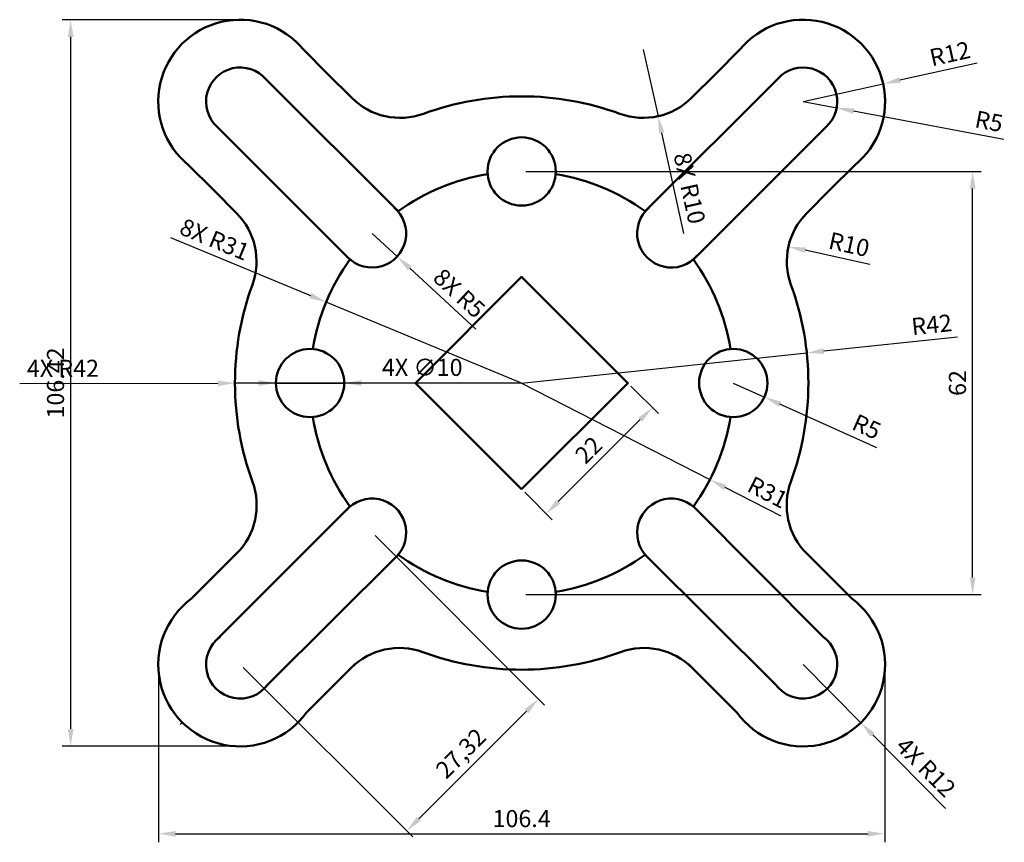
# Model space of a CAD drawing. Units: millimetres. Extents: x 2938 to 3083, y 1829 to 1950.
import ezdxf

# ---------------------------------------------------------------- set-up
doc = ezdxf.new("R2010")
doc.units = ezdxf.units.MM
for name, color, linetype, lineweight in [('M-CONS', 8, 'Continuous', 18), ('M-DIMS', 2, 'Continuous', 25), ('M-OUTL', 7, 'Continuous', 50)]:
    doc.layers.add(name, color=color, linetype=linetype, lineweight=lineweight)
doc.styles.get("Standard").update_dxf_attribs({"font": 'arial.ttf'})
doc.dimstyles.new('ISO-25', dxfattribs={"dimtxt": 2.5, "dimasz": 2.5, "dimexe": 1.25, "dimexo": 0.625, "dimtad": 1, "dimtxsty": 'Standard', "dimcen": 2.5, "dimadec": 0, "dimazin": 0, "dimtfac": 1, "dimtmove": 0, "dimatfit": 3, "dimfxl": 1, "dimarcsym": 0})

# ---------------------------------------------------------------- blocks, each defined once
blk = doc.blocks.new('*D1')
at = {"layer": 'Defpoints', "color": 0, "transparency": 16777216}
for p in [(3027.37, 1896.3), (3011.81, 1880.74), (3015.4, 1877.15)]:
    blk.add_point(p, dxfattribs=at)
at = {"layer": 'M-DIMS', "color": 0, "lineweight": -2, "transparency": 16777216}
for p, q in [((3027.81, 1895.86), (3031.84, 1891.82)), ((3029.19, 1890.94), (3017.17, 1878.92)), ((3012.26, 1880.3), (3016.29, 1876.27))]:
    blk.add_line(p, q, dxfattribs=at)
at = {"layer": 'M-DIMS', "color": 0, "transparency": 16777216}
for points in [[(3028.9, 1891.23), (3029.49, 1890.64), (3030.96, 1892.71)], [(3016.88, 1879.21), (3017.47, 1878.62), (3015.4, 1877.15)]]:
    blk.add_solid(points, dxfattribs=at)
at = {"layer": 'M-DIMS', "color": 0, "transparency": 16777216, "insert": (3021.85, 1886.26), "char_height": 2.5, "attachment_point": 5, "rotation": 45}
blk.add_mtext('22', dxfattribs=at)
blk = doc.blocks.new('*D2')
at = {"layer": 'Defpoints', "color": 0, "transparency": 16777216}
for p in [(3042.81, 1896.3), (3047.37, 1894.24)]:
    blk.add_point(p, dxfattribs=at)
at = {"layer": 'M-DIMS', "color": 0, "lineweight": -2, "transparency": 16777216}
for p, q in [((3042.81, 1896.3), (3047.37, 1894.24)), ((3063.85, 1886.79), (3049.65, 1893.21))]:
    blk.add_line(p, q, dxfattribs=at)
at = {"layer": 'M-DIMS', "color": 0, "transparency": 16777216}
blk.add_solid([(3049.82, 1893.59), (3049.48, 1892.83), (3047.37, 1894.24)], dxfattribs=at)
at = {"layer": 'M-DIMS', "color": 0, "transparency": 16777216, "insert": (3062.22, 1889.61), "char_height": 2.5, "attachment_point": 5, "rotation": 335.6831}
blk.add_mtext('R5', dxfattribs=at)
blk = doc.blocks.new('*D3')
at = {"layer": 'Defpoints', "color": 0, "transparency": 16777216}
for p in [(3053.58, 1900.71), (3011.81, 1896.3)]:
    blk.add_point(p, dxfattribs=at)
at = {"layer": 'M-DIMS', "color": 0, "lineweight": -2, "transparency": 16777216}
for p, q in [((3075.68, 1903.04), (3056.07, 1900.97)), ((3011.81, 1896.3), (3053.58, 1900.71))]:
    blk.add_line(p, q, dxfattribs=at)
at = {"layer": 'M-DIMS', "color": 0, "transparency": 16777216}
blk.add_solid([(3056.02, 1901.39), (3056.11, 1900.56), (3053.58, 1900.71)], dxfattribs=at)
at = {"layer": 'M-DIMS', "color": 0, "transparency": 16777216, "insert": (3071.91, 1904.53), "char_height": 2.5, "attachment_point": 5, "rotation": 6.0281}
blk.add_mtext('R42', dxfattribs=at)
blk = doc.blocks.new('*D4')
at = {"layer": 'Defpoints', "color": 0, "transparency": 16777216}
for p in [(3064.77, 1940.13), (3053.05, 1937.53)]:
    blk.add_point(p, dxfattribs=at)
at = {"layer": 'M-DIMS', "color": 0, "lineweight": -2, "transparency": 16777216}
for p, q in [((3078.53, 1943.18), (3067.21, 1940.67)), ((3053.05, 1937.53), (3064.77, 1940.13))]:
    blk.add_line(p, q, dxfattribs=at)
at = {"layer": 'M-DIMS', "color": 0, "transparency": 16777216}
blk.add_solid([(3067.12, 1941.08), (3067.3, 1940.27), (3064.77, 1940.13)], dxfattribs=at)
at = {"layer": 'M-DIMS', "color": 0, "transparency": 16777216, "insert": (3074.61, 1944.24), "char_height": 2.5, "attachment_point": 5, "rotation": 12.5029}
blk.add_mtext('R12', dxfattribs=at)
blk = doc.blocks.new('*D5')
at = {"layer": 'Defpoints', "color": 0, "transparency": 16777216}
for p in [(3053.05, 1937.53), (3057.96, 1936.61)]:
    blk.add_point(p, dxfattribs=at)
at = {"layer": 'M-DIMS', "color": 0, "lineweight": -2, "transparency": 16777216}
for p, q in [((3053.05, 1937.53), (3057.96, 1936.61)), ((3082.47, 1931.98), (3060.42, 1936.14))]:
    blk.add_line(p, q, dxfattribs=at)
at = {"layer": 'M-DIMS', "color": 0, "transparency": 16777216}
blk.add_solid([(3060.5, 1936.55), (3060.34, 1935.73), (3057.96, 1936.61)], dxfattribs=at)
at = {"layer": 'M-DIMS', "color": 0, "transparency": 16777216, "insert": (3080.22, 1934.33), "char_height": 2.5, "attachment_point": 5, "rotation": 349.3058}
blk.add_mtext('R5', dxfattribs=at)
blk = doc.blocks.new('*D6')
at = {"layer": 'Defpoints', "color": 0, "transparency": 16777216}
for p in [(3011.81, 1896.3), (3039.39, 1882.14)]:
    blk.add_point(p, dxfattribs=at)
at = {"layer": 'M-DIMS', "color": 0, "lineweight": -2, "transparency": 16777216}
for p, q in [((3011.81, 1896.3), (3039.39, 1882.14)), ((3049.84, 1876.78), (3041.61, 1881))]:
    blk.add_line(p, q, dxfattribs=at)
at = {"layer": 'M-DIMS', "color": 0, "transparency": 16777216}
blk.add_solid([(3041.8, 1881.37), (3041.42, 1880.63), (3039.39, 1882.14)], dxfattribs=at)
at = {"layer": 'M-DIMS', "color": 0, "transparency": 16777216, "insert": (3047.71, 1880.01), "char_height": 2.5, "attachment_point": 5, "rotation": 332.822}
blk.add_mtext('R31', dxfattribs=at)
blk = doc.blocks.new('*D7')
at = {"layer": 'Defpoints', "color": 0, "transparency": 16777216}
for p in [(3050.9, 1916.29), (3060.66, 1914.13)]:
    blk.add_point(p, dxfattribs=at)
at = {"layer": 'M-DIMS', "color": 0, "lineweight": -2, "transparency": 16777216}
blk.add_line((3062.82, 1913.65), (3053.34, 1915.75), dxfattribs=at)
at = {"layer": 'M-DIMS', "color": 0, "transparency": 16777216}
blk.add_solid([(3053.43, 1916.16), (3053.25, 1915.34), (3050.9, 1916.29)], dxfattribs=at)
at = {"layer": 'M-DIMS', "color": 0, "transparency": 16777216, "insert": (3059.71, 1916.29), "char_height": 2.5, "attachment_point": 5, "rotation": 347.5289}
blk.add_mtext('R10', dxfattribs=at)
blk = doc.blocks.new('*D8')
at = {"layer": 'Defpoints', "color": 0, "transparency": 16777216}
for p in [(2989.89, 1874.38), (2970.58, 1855.06), (2994.97, 1830.67)]:
    blk.add_point(p, dxfattribs=at)
at = {"layer": 'M-DIMS', "color": 0, "lineweight": -2, "transparency": 16777216}
for p, q in [((2990.33, 1873.94), (3015.17, 1849.1)), ((2971.02, 1854.62), (2995.85, 1829.79)), ((3012.51, 1848.22), (2996.73, 1832.44))]:
    blk.add_line(p, q, dxfattribs=at)
at = {"layer": 'M-DIMS', "color": 0, "transparency": 16777216}
for points in [[(3012.22, 1848.52), (3012.81, 1847.93), (3014.28, 1849.99)], [(2996.44, 1832.73), (2997.03, 1832.15), (2994.97, 1830.67)]]:
    blk.add_solid(points, dxfattribs=at)
at = {"layer": 'M-DIMS', "color": 0, "transparency": 16777216, "insert": (3003.12, 1841.83), "char_height": 2.5, "width": 8.4533, "attachment_point": 5, "rotation": 45}
blk.add_mtext('27,32', dxfattribs=at)
blk = doc.blocks.new('MOUNT-HOLE-D10')
blk.add_circle((5, 5), 5)
blk = doc.blocks.new('*D10')
at = {"layer": 'Defpoints', "color": 0, "transparency": 16777216}
for p in [(2958.61, 1855.96), (3065.02, 1855.96), (3065.02, 1830.26)]:
    blk.add_point(p, dxfattribs=at)
at = {"layer": 'M-DIMS', "color": 0, "lineweight": -2, "transparency": 16777216}
for p, q in [((2958.61, 1855.34), (2958.61, 1829.01)), ((3065.02, 1855.34), (3065.02, 1829.01)), ((2961.11, 1830.26), (3062.52, 1830.26))]:
    blk.add_line(p, q, dxfattribs=at)
at = {"layer": 'M-DIMS', "color": 0, "transparency": 16777216}
for points in [[(2961.11, 1830.67), (2961.11, 1829.84), (2958.61, 1830.26)], [(3062.52, 1830.67), (3062.52, 1829.84), (3065.02, 1830.26)]]:
    blk.add_solid(points, dxfattribs=at)
at = {"layer": 'M-DIMS', "color": 0, "transparency": 16777216, "insert": (3011.81, 1832.16), "char_height": 2.5, "attachment_point": 5}
blk.add_mtext('106.4', dxfattribs=at)
blk = doc.blocks.new('*D11')
at = {"layer": 'Defpoints', "color": 0, "transparency": 16777216}
for p in [(2945.75, 1949.52), (2971.16, 1949.52), (2971.61, 1843.11)]:
    blk.add_point(p, dxfattribs=at)
at = {"layer": 'M-DIMS', "color": 0, "lineweight": -2, "transparency": 16777216}
for p, q in [((2970.54, 1949.52), (2944.5, 1949.52)), ((2945.75, 1845.61), (2945.75, 1947.02)), ((2970.98, 1843.11), (2944.5, 1843.11))]:
    blk.add_line(p, q, dxfattribs=at)
at = {"layer": 'M-DIMS', "color": 0, "transparency": 16777216}
for points in [[(2945.33, 1947.02), (2946.16, 1947.02), (2945.75, 1949.52)], [(2945.33, 1845.61), (2946.16, 1845.61), (2945.75, 1843.11)]]:
    blk.add_solid(points, dxfattribs=at)
at = {"layer": 'M-DIMS', "color": 0, "transparency": 16777216, "insert": (2943.85, 1896.31), "char_height": 2.5, "attachment_point": 5, "rotation": 90}
blk.add_mtext('106.42', dxfattribs=at)
blk = doc.blocks.new('*D12')
at = {"layer": 'Defpoints', "color": 0, "transparency": 16777216}
for p in [(3011.81, 1927.3), (3077.88, 1927.3), (3011.81, 1865.3)]:
    blk.add_point(p, dxfattribs=at)
at = {"layer": 'M-DIMS', "color": 0, "lineweight": -2, "transparency": 16777216}
for p, q in [((3012.44, 1927.3), (3079.13, 1927.3)), ((3077.88, 1867.8), (3077.88, 1924.8)), ((3012.44, 1865.3), (3079.13, 1865.3))]:
    blk.add_line(p, q, dxfattribs=at)
at = {"layer": 'M-DIMS', "color": 0, "transparency": 16777216}
for points in [[(3077.46, 1924.8), (3078.3, 1924.8), (3077.88, 1927.3)], [(3077.46, 1867.8), (3078.3, 1867.8), (3077.88, 1865.3)]]:
    blk.add_solid(points, dxfattribs=at)
at = {"layer": 'M-DIMS', "color": 0, "transparency": 16777216, "insert": (3075.98, 1896.3), "char_height": 2.5, "attachment_point": 5, "rotation": 90}
blk.add_mtext('62', dxfattribs=at)
blk = doc.blocks.new('*D13')
at = {"layer": 'Defpoints', "color": 0, "transparency": 16777216}
for p in [(2969.81, 1896.27), (3011.81, 1896.3)]:
    blk.add_point(p, dxfattribs=at)
at = {"layer": 'M-DIMS', "color": 0, "lineweight": -2, "transparency": 16777216}
for p, q in [((2938.28, 1896.25), (2967.31, 1896.27)), ((3011.81, 1896.3), (2969.81, 1896.27))]:
    blk.add_line(p, q, dxfattribs=at)
at = {"layer": 'M-DIMS', "color": 0, "transparency": 16777216}
blk.add_solid([(2967.31, 1896.68), (2967.31, 1895.85), (2969.81, 1896.27)], dxfattribs=at)
at = {"layer": 'M-DIMS', "color": 0, "transparency": 16777216, "insert": (2944.61, 1898.13), "char_height": 2.5, "attachment_point": 5, "rotation": 0.0393}
blk.add_mtext('4X R42', dxfattribs=at)
blk = doc.blocks.new('*D14')
at = {"layer": 'Defpoints', "color": 0, "transparency": 16777216}
for p in [(2983.17, 1908.16), (3011.81, 1896.3)]:
    blk.add_point(p, dxfattribs=at)
at = {"layer": 'M-DIMS', "color": 0, "lineweight": -2, "transparency": 16777216}
for p, q in [((2960.39, 1917.6), (2980.86, 1909.12)), ((3011.81, 1896.3), (2983.17, 1908.16))]:
    blk.add_line(p, q, dxfattribs=at)
at = {"layer": 'M-DIMS', "color": 0, "transparency": 16777216}
blk.add_solid([(2981.02, 1909.5), (2980.7, 1908.73), (2983.17, 1908.16)], dxfattribs=at)
at = {"layer": 'M-DIMS', "color": 0, "transparency": 16777216, "insert": (2966.72, 1917.04), "char_height": 2.5, "attachment_point": 5, "rotation": 337.4999}
blk.add_mtext('8X R31', dxfattribs=at)
blk = doc.blocks.new('*D15')
at = {"layer": 'Defpoints', "color": 0, "transparency": 16777216}
for p in [(3053.05, 1855.06), (3061.49, 1846.53)]:
    blk.add_point(p, dxfattribs=at)
at = {"layer": 'M-DIMS', "color": 0, "lineweight": -2, "transparency": 16777216}
for p, q in [((3053.05, 1855.06), (3061.49, 1846.53)), ((3073.92, 1833.97), (3063.25, 1844.75))]:
    blk.add_line(p, q, dxfattribs=at)
at = {"layer": 'M-DIMS', "color": 0, "transparency": 16777216}
blk.add_solid([(3063.54, 1845.05), (3062.95, 1844.46), (3061.49, 1846.53)], dxfattribs=at)
at = {"layer": 'M-DIMS', "color": 0, "transparency": 16777216, "insert": (3070.8, 1839.79), "char_height": 2.5, "attachment_point": 5, "rotation": 314.6894}
blk.add_mtext('4X R12', dxfattribs=at)
blk = doc.blocks.new('*D16')
at = {"layer": 'Defpoints', "color": 0, "transparency": 16777216}
for p in [(3029.63, 1945.15), (3031.79, 1935.39)]:
    blk.add_point(p, dxfattribs=at)
at = {"layer": 'M-DIMS', "color": 0, "lineweight": -2, "transparency": 16777216}
for p, q in [((3029.63, 1945.15), (3031.79, 1935.39)), ((3035.59, 1918.21), (3032.33, 1932.94))]:
    blk.add_line(p, q, dxfattribs=at)
at = {"layer": 'M-DIMS', "color": 0, "transparency": 16777216}
blk.add_solid([(3032.74, 1933.03), (3031.93, 1932.85), (3031.79, 1935.39)], dxfattribs=at)
at = {"layer": 'M-DIMS', "color": 0, "transparency": 16777216, "insert": (3036.09, 1924.77), "char_height": 2.5, "attachment_point": 5, "rotation": 282.4775}
blk.add_mtext('8X R10', dxfattribs=at)
blk = doc.blocks.new('*D17')
at = {"layer": 'Defpoints', "color": 0, "transparency": 16777216}
for p in [(2989.89, 1918.22), (2993.57, 1914.83)]:
    blk.add_point(p, dxfattribs=at)
at = {"layer": 'M-DIMS', "color": 0, "lineweight": -2, "transparency": 16777216}
for p, q in [((2989.89, 1918.22), (2993.57, 1914.83)), ((3005.09, 1904.2), (2995.41, 1913.13))]:
    blk.add_line(p, q, dxfattribs=at)
at = {"layer": 'M-DIMS', "color": 0, "transparency": 16777216}
blk.add_solid([(2995.69, 1913.44), (2995.12, 1912.83), (2993.57, 1914.83)], dxfattribs=at)
at = {"layer": 'M-DIMS', "color": 0, "transparency": 16777216, "insert": (3002.46, 1909.22), "char_height": 2.5, "attachment_point": 5, "rotation": 317.31}
blk.add_mtext('8X R5', dxfattribs=at)
blk = doc.blocks.new('*D18')
at = {"layer": 'Defpoints', "color": 0, "transparency": 16777216}
for p in [(2975.81, 1896.3), (2985.81, 1896.3)]:
    blk.add_point(p, dxfattribs=at)
at = {"layer": 'M-DIMS', "color": 0, "lineweight": -2, "transparency": 16777216}
for p, q in [((2973.31, 1896.3), (2970.81, 1896.3)), ((2975.81, 1896.3), (2985.81, 1896.3)), ((3003.7, 1896.3), (2988.31, 1896.3))]:
    blk.add_line(p, q, dxfattribs=at)
at = {"layer": 'M-DIMS', "color": 0, "transparency": 16777216}
for points in [[(2973.31, 1896.71), (2973.31, 1895.88), (2975.81, 1896.3)], [(2988.31, 1896.71), (2988.31, 1895.88), (2985.81, 1896.3)]]:
    blk.add_solid(points, dxfattribs=at)
at = {"layer": 'M-DIMS', "color": 0, "transparency": 16777216, "insert": (2997.25, 1898.27), "char_height": 2.5, "attachment_point": 5, "rotation": 0.0023}
blk.add_mtext('4X ∅10', dxfattribs=at)

msp = doc.modelspace()

# ---------------------------------------------------------------- linework, layer by layer
at = {"layer": 'M-CONS'}
for p, q in [((2961.8, 1846.284), (2962.091, 1846.576)), ((2962.091, 1846.576), (2961.8, 1846.284))]:
    msp.add_line(p, q, dxfattribs=at)
at = {"layer": 'M-OUTL'}
for p, q in [((2979.853, 1945.147), (2983.388, 1941.612)), ((3043.774, 1945.147), (3040.238, 1941.612)), ((2983.388, 1941.612), (2986.924, 1938.076)), ((3040.238, 1941.612), (3036.703, 1938.076)), ((2993.702, 1921.457), (2974.386, 1940.773)), ((3049.384, 1940.934), (3029.924, 1921.457)), ((2967.217, 1933.831), (2986.357, 1914.683)), ((3036.972, 1914.409), (3056.409, 1933.831)), ((2963.066, 1928.175), (2966.601, 1924.64)), ((3060.56, 1928.175), (3057.025, 1924.64)), ((2966.601, 1924.64), (2970.137, 1921.104)), ((3057.025, 1924.64), (3053.489, 1921.104)), ((2986.654, 1878.187), (2967.043, 1858.599)), ((3036.972, 1878.187), (3055.958, 1859.128)), ((2963.457, 1864.721), (2970.528, 1871.792)), ((2974.675, 1852.197), (2993.418, 1870.832)), ((3048.951, 1852.197), (3030.208, 1870.832)), ((3060.169, 1864.721), (3053.098, 1871.792)), ((2980.313, 1848.047), (2987.384, 1855.118)), ((3043.313, 1848.047), (3036.242, 1855.118))]:
    msp.add_line(p, q, dxfattribs=at)
msp.add_lwpolyline([(3011.813, 1880.741), (2996.257, 1896.298), (3011.813, 1911.854), (3027.37, 1896.298)], close=True, dxfattribs=at)
for centre, radius, start, end in [((2970.577, 1937.534), 12, 39.37648, 231.25202), ((3053.05, 1937.534), 12, 308.74798, 140.62352), ((2970.577, 1937.534), 5, 40.37435, 227.78466), ((3053.05, 1937.534), 5, 312.21534, 137.15616), ((2993.993, 1945.149), 10, 225, 290.04121), ((3011.813, 1896.298), 42, 69.95879, 110.04121), ((3029.633, 1945.149), 10, 249.95879, 315), ((3011.813, 1896.298), 31, 99.2513, 125.7487), ((3011.813, 1896.298), 31, 54.2513, 80.7487), ((2989.893, 1918.218), 5, 224.98751, 49.62565), ((3033.734, 1918.218), 5, 130.4274, 319.58236), ((2962.967, 1914.132), 10, 339.94224, 45), ((3060.659, 1914.132), 10, 135, 200.05776), ((3011.813, 1896.298), 31, 144.2513, 170.7487), ((3011.813, 1896.298), 31, 9.2513, 35.7487), ((3011.813, 1896.298), 42, 159.94224, 200.13531), ((3011.813, 1896.298), 42, 339.86469, 20.05776), ((3011.813, 1896.298), 31, 189.2513, 215.7487), ((3011.813, 1896.298), 31, 324.2513, 350.7487), ((2962.991, 1878.397), 10, 315, 20.13531), ((3060.635, 1878.397), 10, 159.86469, 225), ((2989.893, 1874.377), 5, 314.83368, 139.55833), ((3033.734, 1874.377), 5, 40.15592, 225.16632), ((3011.813, 1896.298), 31, 234.2513, 260.7487), ((3011.813, 1896.298), 31, 279.2513, 305.7487), ((2970.577, 1855.061), 12, 126.39081, 324.23086), ((3053.05, 1855.061), 12, 215.76914, 53.60919), ((2970.577, 1855.061), 5, 125.57027, 325.05141), ((3053.05, 1855.061), 5, 214.94859, 54.42973), ((2993.892, 1847.484), 10, 69.84017, 135), ((3011.813, 1896.298), 42, 249.84017, 290.15983), ((3029.734, 1847.484), 10, 45, 110.15983)]:
    msp.add_arc(centre, radius, start, end, dxfattribs=at)

# ---------------------------------------------------------------- block references
for p in [(3006.813, 1922.298), (2975.813, 1891.298), (3037.813, 1891.298), (3006.813, 1860.298)]:
    msp.add_blockref('MOUNT-HOLE-D10', p, dxfattribs=at)

# ---------------------------------------------------------------- dimensions: what is measured, and where the dimension line sits
at = {"layer": 'M-DIMS'}
for base, p1, p2, override, picture, middle in [((2945.74782, 1949.52034), (2971.60894, 1843.10528), (2971.16381, 1949.52034), {"dimdec": 2, "dimlfac": 1, "dimrnd": 0, "dimzin": 0, "dimdsep": 46, "dimlunit": 2}, '*D11', (2943.84639, 1896.31281)), ((3077.879, 1927.298), (3011.813, 1865.298), (3011.813, 1927.298), {"dimdec": 0, "dimlfac": 1, "dimrnd": 0, "dimzin": 0, "dimdsep": 46, "dimlunit": 2}, '*D12', (3075.977, 1896.298))]:
    dim = msp.add_linear_dim(base=base, p1=p1, p2=p2, angle=90, dimstyle='ISO-25', override=override, dxfattribs=at)
    dim.commit()
    dim.dimension.update_dxf_attribs({"geometry": picture, "text_midpoint": middle})
for center, mpoint, picture, middle in [((3053.05, 1937.534), (3064.765, 1940.132), '*D4', (3075.016, 1942.405)), ((3053.05, 1937.534), (3057.963, 1936.606), '*D5', (3079.866, 1932.47)), ((3060.659, 1914.132), (3050.895, 1916.292), '*D7', (3059.3, 1914.433)), ((3011.813, 1896.298), (3053.581, 1900.709), '*D3', (3072.106, 1902.665)), ((3042.813, 1896.298), (3047.37, 1894.239), '*D2', (3061.435, 1887.883))]:
    dim = msp.add_radius_dim(center=center, mpoint=mpoint, dimstyle='ISO-25', override={"dimclrd": 0, "dimclre": 0, "dimclrt": 0}, dxfattribs=at)
    dim.commit()
    dim.dimension.update_dxf_attribs({"geometry": picture, "text_midpoint": middle, "dimtype": 164})
for center, mpoint, text, picture, middle in [((3029.633, 1945.149), (3031.794, 1935.385), '8X <>', '*D16', (3036.091, 1924.768)), ((2989.893, 1918.218), (2993.568, 1914.828), '8X <>', '*D17', (3002.456, 1909.216)), ((3053.05, 1855.061), (3061.489, 1846.53), '4X <>', '*D15', (3070.798, 1839.794))]:
    dim = msp.add_radius_dim(center=center, mpoint=mpoint, text=text, dimstyle='ISO-25', override={"dimdec": 0, "dimlfac": 1, "dimrnd": 0, "dimzin": 0, "dimdsep": 46, "dimlunit": 2}, dxfattribs=at)
    dim.commit()
    dim.dimension.update_dxf_attribs({"geometry": picture, "text_midpoint": middle})
for mpoint, text, picture, middle in [((2983.173, 1908.161), '8X <>', '*D14', (2965.989, 1915.279)), ((2969.813, 1896.269), '4X <>', '*D13', (2944.613, 1896.252))]:
    dim = msp.add_radius_dim(center=(3011.813, 1896.298), mpoint=mpoint, text=text, dimstyle='ISO-25', override={"dimdec": 0, "dimlfac": 1, "dimrnd": 0, "dimzin": 0, "dimdsep": 46, "dimlunit": 2}, dxfattribs=at)
    dim.commit()
    dim.dimension.update_dxf_attribs({"geometry": picture, "text_midpoint": middle, "dimtype": 164})
dim = msp.add_diameter_dim_2p(p1=(2975.813, 1896.298), p2=(2985.813, 1896.298), text='4X <>', dimstyle='ISO-25', override={"dimdec": 0, "dimlfac": 1, "dimrnd": 0, "dimzin": 0, "dimdsep": 46, "dimlunit": 2}, dxfattribs=at)
dim.commit()
dim.dimension.update_dxf_attribs({"geometry": '*D18', "text_midpoint": (2997.254, 1896.298)})
for p1, p2, distance, picture, middle in [((3027.37, 1896.298), (3011.813, 1880.741), 5.078, '*D1', (3021.853, 1886.258)), ((2989.893, 1874.377), (2970.577, 1855.061), 34.491, '*D8', (3003.12, 1841.835))]:
    dim = msp.add_aligned_dim(p1=p1, p2=p2, distance=distance, dimstyle='ISO-25', override={"dimclrd": 0, "dimclre": 0, "dimclrt": 0}, dxfattribs=at)
    dim.commit()
    dim.dimension.update_dxf_attribs({"geometry": picture, "text_midpoint": middle})
dim = msp.add_radius_dim(center=(3011.813, 1896.298), mpoint=(3039.391, 1882.138), dimstyle='ISO-25', override={"dimclrd": 0, "dimclre": 0, "dimclrt": 0}, dxfattribs=at)
dim.commit()
dim.dimension.update_dxf_attribs({"geometry": '*D6', "text_midpoint": (3047.706, 1880.007)})
dim = msp.add_linear_dim(base=(3065.016, 1830.255), p1=(2958.61, 1855.964), p2=(3065.016, 1855.964), dimstyle='ISO-25', override={"dimdec": 1, "dimlfac": 1, "dimrnd": 0, "dimzin": 0, "dimdsep": 46, "dimlunit": 2}, dxfattribs=at)
dim.commit()
dim.dimension.update_dxf_attribs({"geometry": '*D10', "text_midpoint": (3011.813, 1832.157)})

doc.saveas('drawing.dxf')
